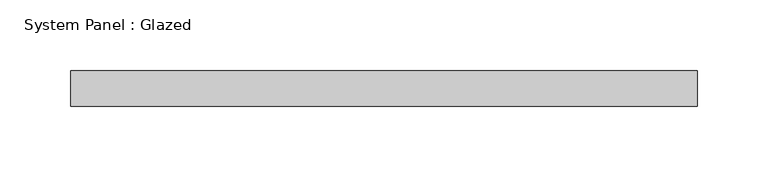
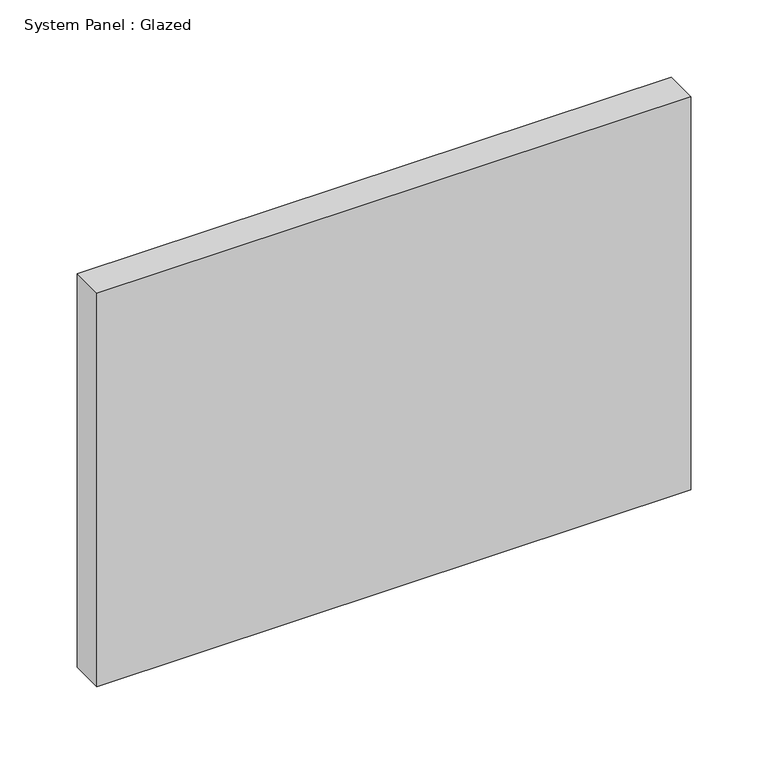
"""IFC4 building model written with IfcOpenShell, lengths in millimetres: plate geometry, System Panel : Glazed."""

from ifc_helpers import new_model, si_unit, origin, origin_with_axes, place, context, project, spatial, polyline, outline, extrude, source, transform, mapped, element, save


def system_panel_glazed_145a7978(model_context):
    return source(origin(), model_context, "Body", "SweptSolid", [
        extrude(outline(polyline([(222.25, 19.05), (-222.25, 19.05), (-222.25, 44.45), (222.25, 44.45), (222.25, 19.05)])), origin_with_axes(), (0.0, 0.0, 1.0), 311.15),
    ])


if __name__ == "__main__":
    model = new_model("IFC4")
    model_context = context("Model", 3, world=origin())
    ifc_project = project(units=[si_unit("LENGTHUNIT", "METRE", prefix="MILLI")], contexts=[model_context])
    site = spatial("IfcSite", under=ifc_project)
    building = spatial("IfcBuilding", under=site)
    placement = place(None, origin())
    system_panel_glazed_shape = system_panel_glazed_145a7978(model_context)
    element("IfcPlate", 1, ObjectType="System Panel : Glazed", at=placement, inside=building, context=model_context, shape_type="MappedRepresentation", body=[
        mapped(system_panel_glazed_shape, transform((0.0, 0.0, 0.0), x_axis=(1.0, 0.0, 0.0), y_axis=(0.0, 1.0, 0.0), z_axis=(0.0, 0.0, 1.0))),
    ])
    save(model, "model.ifc")

# Revit data of these elements
# Type "System Panel : Glazed"
#   Construction Type Id = "GSP4R"
#   Analytic Construction = "1/8 in Pilkington single glazing"
#   Visual Light Transmittance = 0.9
#   Solar Heat Gain Coefficient = 0.86
#   Heat Transfer Coefficient (U) = 1.18115 BTU/(h·ft²·°F)
#   Define Thermal Properties by = 1
# Element 1 (IfcPlate, "System Panel : Glazed")
#   Materials on its faces: "Glass"
# Materials
#   "Glass": class "Glass", colour RGB 0 128 192, transparency 0.75, Description = "Soda Lime Glass", Cost = 0
